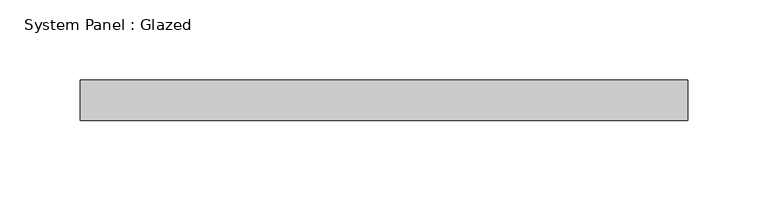
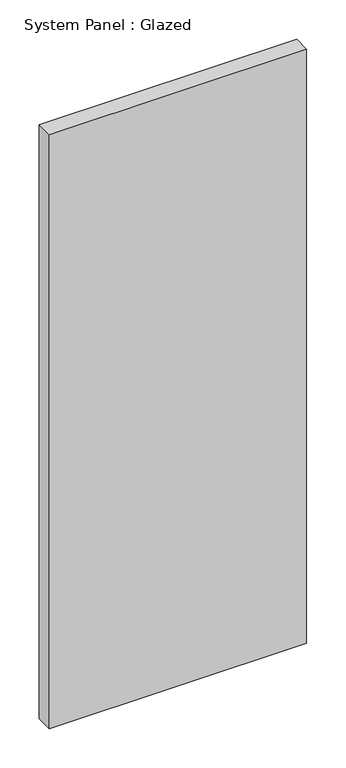
"""IFC4 building model written with IfcOpenShell, lengths in millimetres: plate geometry, System Panel : Glazed."""

from ifc_helpers import new_model, si_unit, origin, origin_with_axes, place, context, project, spatial, polyline, outline, extrude, source, transform, mapped, element, save


def system_panel_glazed_ab35909a(model_context):
    return source(origin(), model_context, "Body", "SweptSolid", [
        extrude(outline(polyline([(189.3828999, 19.05), (-189.3828999, 19.05), (-189.3828999, 44.45), (189.3828999, 44.45), (189.3828999, 19.05)])), origin_with_axes(), (0.0, 0.0, 1.0), 923.1640555),
    ])


if __name__ == "__main__":
    model = new_model("IFC4")
    model_context = context("Model", 3, world=origin())
    ifc_project = project(units=[si_unit("LENGTHUNIT", "METRE", prefix="MILLI")], contexts=[model_context])
    site = spatial("IfcSite", under=ifc_project)
    building = spatial("IfcBuilding", under=site)
    placement = place(None, origin())
    system_panel_glazed_shape = system_panel_glazed_ab35909a(model_context)
    element("IfcPlate", 1, ObjectType="System Panel : Glazed", at=placement, inside=building, context=model_context, shape_type="MappedRepresentation", body=[
        mapped(system_panel_glazed_shape, transform((0.0, 0.0, 0.0), x_axis=(1.0, 0.0, 0.0), y_axis=(0.0, 1.0, 0.0), z_axis=(0.0, 0.0, 1.0))),
    ])
    save(model, "model.ifc")

# Revit data of these elements
# Type "System Panel : Glazed"
#   Construction Type Id = "GSP4R"
#   Analytic Construction = "1/8 in Pilkington single glazing"
#   Visual Light Transmittance = 0.9
#   Solar Heat Gain Coefficient = 0.86
#   Heat Transfer Coefficient (U) = 1.18115 BTU/(h·ft²·°F)
# Element 1 (IfcPlate, "System Panel : Glazed")
#   Materials on its faces: "Glass"
# Materials
#   "Glass": class "Glass", colour RGB 0 128 192, transparency 0.75, Description = "Soda Lime Glass", Cost = 0
